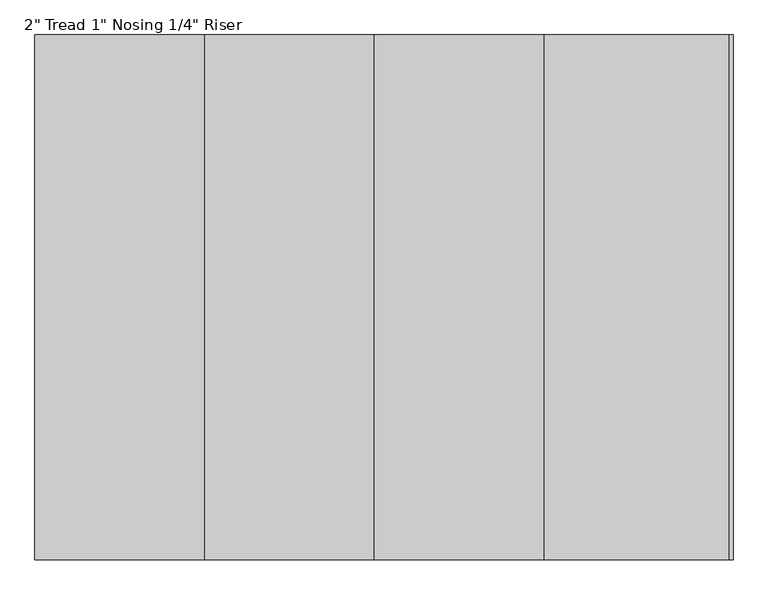
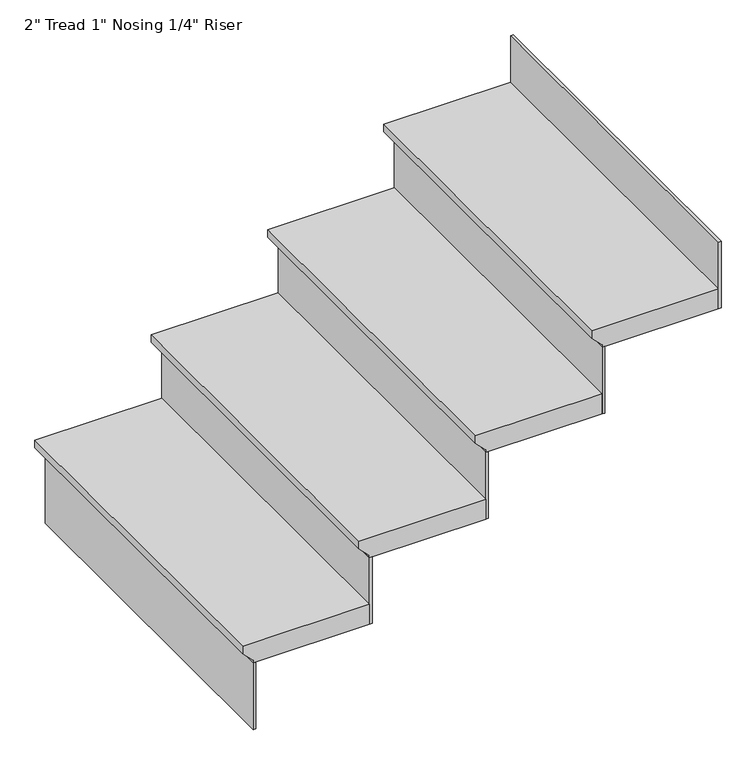
"""IFC4 building model written with IfcOpenShell, lengths in millimetres: stair flight geometry."""

from ifc_helpers import new_model, si_unit, frame, origin, place, context, project, spatial, polyline, outline, extrude, source, transform, mapped, element, save


def stair_flight_c310d209(model_context):
    return source(origin(), model_context, "Body", "SweptSolid", [
        extrude(outline(polyline([(2370.6666667, 4734.0597674), (2370.6666667, 4429.2597674), (2351.6166667, 4429.2597674), (2326.2166667, 4454.6597674), (2319.8666667, 4454.6597674), (2319.8666667, 4734.0597674), (2370.6666667, 4734.0597674)])), frame((0.0, 461.5758265, 0.0), z_axis=(0.0, 1.0, 0.0), x_axis=(0.0, 0.0, 1.0)), (0.0, 0.0, 1.0), 863.6),
        extrude(outline(polyline([(4461.0097674, 461.5758265), (4454.6597674, 461.5758265), (4454.6597674, 1325.1758265), (4461.0097674, 1325.1758265), (4461.0097674, 461.5758265)])), frame((0.0, 0.0, 2150.5333333), z_axis=(0.0, 0.0, 1.0), x_axis=(1.0, 0.0, 0.0)), (0.0, 0.0, 1.0), 169.3333333),
        extrude(outline(polyline([(4740.4097674, 461.5758265), (4734.0597674, 461.5758265), (4734.0597674, 1325.1758265), (4740.4097674, 1325.1758265), (4740.4097674, 461.5758265)])), frame((0.0, 0.0, 2319.8666667), z_axis=(0.0, 0.0, 1.0), x_axis=(1.0, 0.0, 0.0)), (0.0, 0.0, 1.0), 169.3333333),
        extrude(outline(polyline([(2540.0, 5013.4597674), (2540.0, 4708.6597674), (2520.95, 4708.6597674), (2495.55, 4734.0597674), (2489.2, 4734.0597674), (2489.2, 5013.4597674), (2540.0, 5013.4597674)])), frame((0.0, 461.5758265, 0.0), z_axis=(0.0, 1.0, 0.0), x_axis=(0.0, 0.0, 1.0)), (0.0, 0.0, 1.0), 863.6),
        extrude(outline(polyline([(5019.8097674, 461.5758265), (5013.4597674, 461.5758265), (5013.4597674, 1325.1758265), (5019.8097674, 1325.1758265), (5019.8097674, 461.5758265)])), frame((0.0, 0.0, 2489.2), z_axis=(0.0, 0.0, 1.0), x_axis=(1.0, 0.0, 0.0)), (0.0, 0.0, 1.0), 169.3333333),
        extrude(outline(polyline([(2709.3333333, 5292.8597674), (2709.3333333, 4988.0597674), (2690.2833333, 4988.0597674), (2664.8833333, 5013.4597674), (2658.5333333, 5013.4597674), (2658.5333333, 5292.8597674), (2709.3333333, 5292.8597674)])), frame((0.0, 461.5758265, 0.0), z_axis=(0.0, 1.0, 0.0), x_axis=(0.0, 0.0, 1.0)), (0.0, 0.0, 1.0), 863.6),
        extrude(outline(polyline([(5299.2097674, 461.5758265), (5292.8597674, 461.5758265), (5292.8597674, 1325.1758265), (5299.2097674, 1325.1758265), (5299.2097674, 461.5758265)])), frame((0.0, 0.0, 2658.5333333), z_axis=(0.0, 0.0, 1.0), x_axis=(1.0, 0.0, 0.0)), (0.0, 0.0, 1.0), 169.3333333),
        extrude(outline(polyline([(5578.6097674, 461.5758265), (5572.2597674, 461.5758265), (5572.2597674, 1325.1758265), (5578.6097674, 1325.1758265), (5578.6097674, 461.5758265)])), frame((0.0, 0.0, 2827.8666667), z_axis=(0.0, 0.0, 1.0), x_axis=(1.0, 0.0, 0.0)), (0.0, 0.0, 1.0), 169.3333333),
        extrude(outline(polyline([(2878.6666667, 5572.2597674), (2878.6666667, 5267.4597674), (2859.6166667, 5267.4597674), (2834.2166667, 5292.8597674), (2827.8666667, 5292.8597674), (2827.8666667, 5572.2597674), (2878.6666667, 5572.2597674)])), frame((0.0, 461.5758265, 0.0), z_axis=(0.0, 1.0, 0.0), x_axis=(0.0, 0.0, 1.0)), (0.0, 0.0, 1.0), 863.6),
    ])


if __name__ == "__main__":
    model = new_model("IFC4")
    model_context = context("Model", 3, world=origin())
    ifc_project = project(units=[si_unit("LENGTHUNIT", "METRE", prefix="MILLI")], contexts=[model_context])
    site = spatial("IfcSite", under=ifc_project)
    building = spatial("IfcBuilding", under=site)
    placement = place(None, origin())
    stair_flight_shape = stair_flight_c310d209(model_context)
    element("IfcStairFlight", 1, ObjectType="2\" Tread 1\" Nosing 1/4\" Riser", at=placement, inside=building, context=model_context, shape_type="MappedRepresentation", body=[
        mapped(stair_flight_shape, transform((0.0, 0.0, 0.0), x_axis=(1.0, 0.0, 0.0), y_axis=(0.0, 1.0, 0.0), z_axis=(0.0, 0.0, 1.0))),
    ])
    save(model, "model.ifc")
